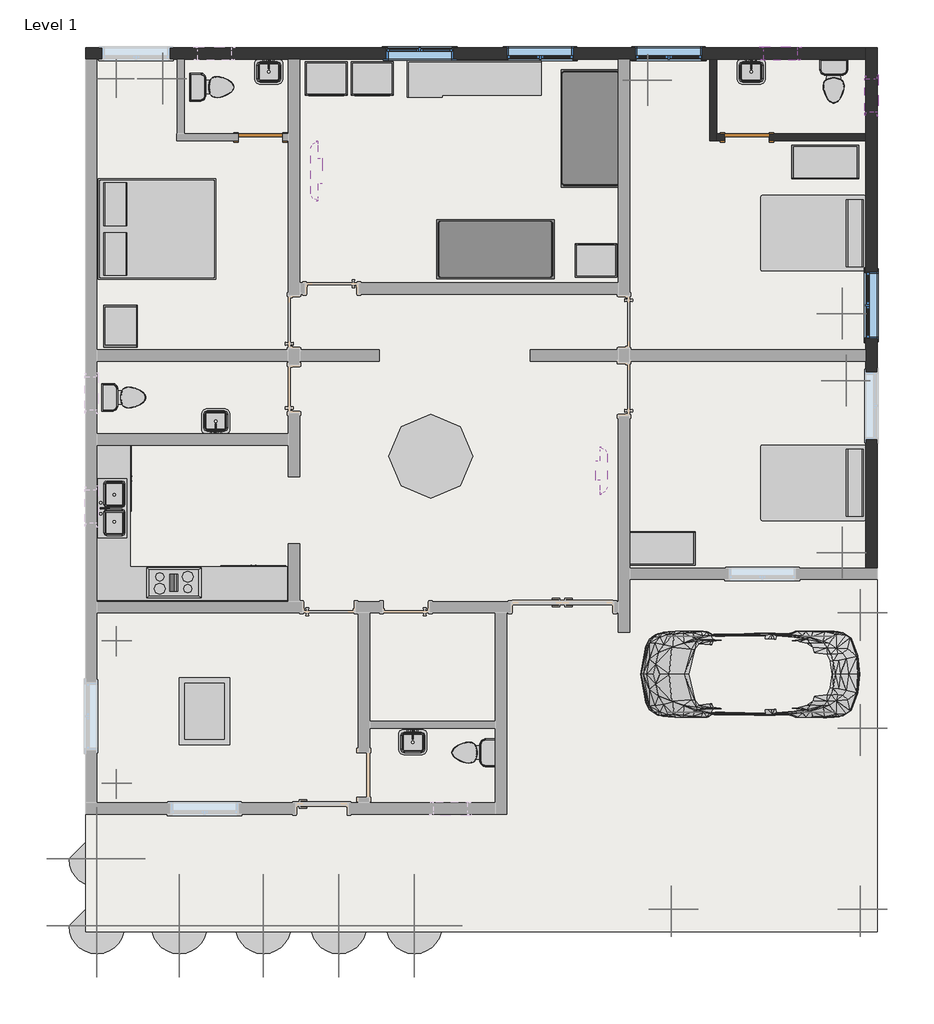
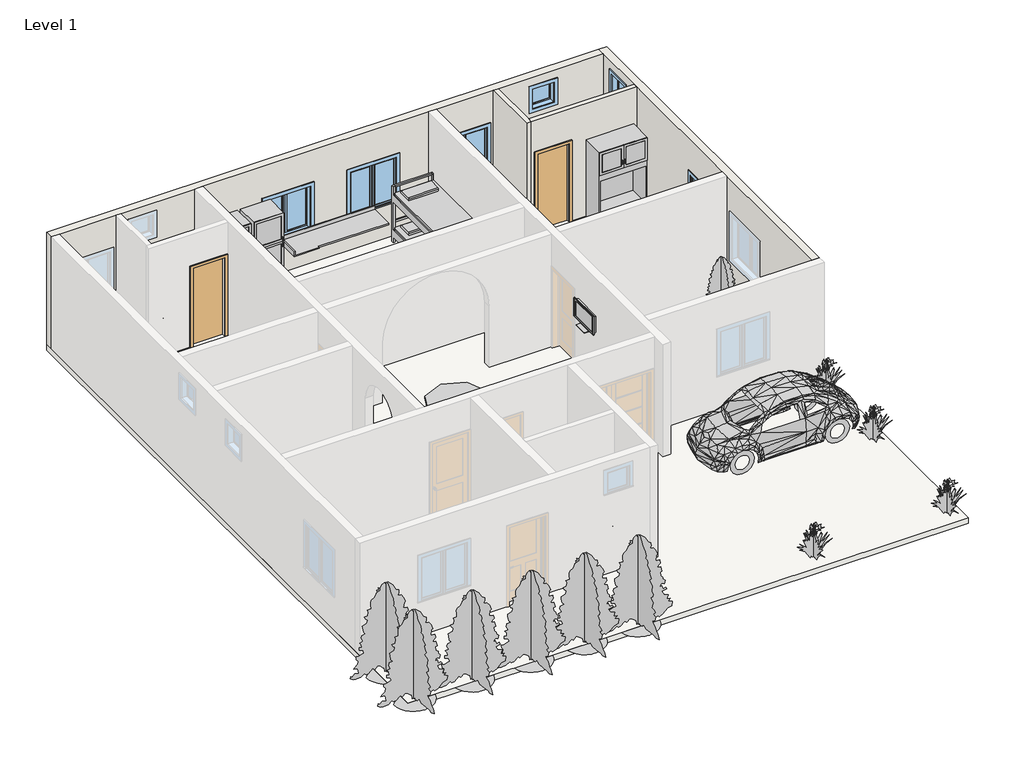
# One storey, part 2 of 2: 20 furniture elements, 18 geographic elements, 9 flow terminals, 6 windows, 4 walls, 2 doors, 2 proxies, 1 slab.
# Revit data of these elements (continued)
# Element 25 (IfcFurniture, "TV - Flat Screen : 42\"")
#   Stand = yes
#   Phase Created = New Construction
#   Materials on its faces: "TV - Black", "TV - Glass", "TV - Screen"
# Element 26 (IfcFurniture, "Table-Coffee : 24\" x 24\" x 24\"")
#   Phase Created = New Construction
#   Materials on its faces: "Glass - Clear, Grey"
# Element 27 (IfcFurniture, "Table-Dining Round w Chairs : 36\" Diameter")
#   Phase Created = New Construction
#   Materials on its faces: "Pine", "Laminate, Linen, Matte"
# Element 28 (IfcFurniture, "Tall Cabinet-2 Door-Built in : 3'")
#   Phase Created = New Construction
#   Materials on its faces: "Cabinets", "Cabinets - Handles", "Glass"
# Elements 29, 30 (IfcFurniture, "Tall Cabinet-2 Door-Built in : 30\"")
#   Phase Created = New Construction
#   Materials on its faces: "Cabinets", "Cabinets - Handles", "Glass"
# Elements 31, 32, 33 (IfcFurniture, "Tall Cabinet-Single Door(2) : 30\"")
#   Phase Created = New Construction
#   Materials on its faces: "Cabinets", "Cabinets - Handles"
# Elements 34, 35, 36, 37 (IfcGeographicElement, "RPC Plant - Tropical")
#   Phase Created = New Construction
# Elements 38, 39, 40, 41, 42, 43 (IfcGeographicElement, "RPC Tree - Conifer")
#   Phase Created = New Construction
# Element 44 (IfcGeographicElement, "RPC Tree - Conifer : 8'")
#   Phase Created = New Construction
# Elements 45, 46 (IfcGeographicElement, "RPC Tree - Conifer : Chinese Juniper - 7'")
#   Phase Created = New Construction
# Element 47 (IfcGeographicElement, "RPC Tree - Conifer : Eastern Hemlock - 25'")
#   Phase Created = New Construction
# Element 48 (IfcGeographicElement, "RPC Tree - Conifer : r")
#   Phase Created = New Construction
# Elements 49, 50 (IfcGeographicElement, "RPC Tree - Conifer : t")
#   Phase Created = New Construction
# Element 51 (IfcGeographicElement, "RPC Tree - Conifer : y")
#   Phase Created = New Construction
# Element 52 (IfcSlab, "Generic - 12\"")
#   Height Offset From Level = 0' - 0"
#   Phase Created = New Construction
#   Materials on its faces: "Oak Flooring"
# Elements 53, 54 (IfcWall, "Generic - 5\"")
#   Top Offset = 0' - 0"
#   Base Offset = 0' - 0"
#   Unconnected Height = 10' - 0"
#   wall height = 10' - 0"
#   Phase Created = New Construction
#   Base Constraint = Level 1
#   Materials on its faces: "Default Wall"
# Element 55 (IfcWall, "Generic - 8\"")
#   Top Offset = 0' - 0"
#   Base Offset = 0' - 0"
#   Unconnected Height = 10' - 0"
#   wall height = 10' - 0"
#   Phase Created = New Construction
#   Base Constraint = Level 1
#   Materials on its faces: "Paint - Sienna", "Default Wall"
# Element 56 (IfcWall, "Generic - 8\"")
#   Top Offset = 0' - 0"
#   Base Offset = 0' - 0"
#   Unconnected Height = 10' - 0"
#   wall height = 10' - 0"
#   Phase Created = New Construction
#   Base Constraint = Level 1
#   Materials on its faces: "Paint - Sienna"
# Element 57 (IfcWindow, "Casement Dbl with Trim : 48\" x 48\"")
#   Mark = "2"
#   Phase Created = New Construction
#   Materials on its faces: "Sash", "Trim", "Glass"
# Element 58 (IfcWindow, "Casement Dbl with Trim : 48\" x 48\"")
#   Mark = "3"
#   Phase Created = New Construction
#   Materials on its faces: "Sash", "Trim", "Glass"
# Element 59 (IfcWindow, "Casement Dbl with Trim : 48\" x 48\"")
#   Mark = "4"
#   Phase Created = New Construction
#   Materials on its faces: "Sash", "Trim", "Glass"
# Element 60 (IfcWindow, "Casement Dbl with Trim : 48\" x 48\"")
#   Mark = "5"
#   Phase Created = New Construction
#   Materials on its faces: "Sash", "Trim", "Glass"
# Element 61 (IfcWindow, "Transom with Trim : 24\" x 24\"")
#   Mark = "12"
#   Phase Created = New Construction
#   Materials on its faces: "Sash", "Trim", "Glass"
# Element 62 (IfcWindow, "Transom with Trim : 24\" x 24\"")
#   Mark = "13"
#   Phase Created = New Construction
#   Materials on its faces: "Sash", "Trim", "Glass"
# Materials
#   "Steel, Chrome Plated": class "Metal", colour RGB 17 17 17, transparency 0, Description = "Chromiuim plated steel", Cost = 0
#   "Steel, Polished": class "Metal", colour RGB 192 192 192, transparency 0, Description = "Polished steel", Cost = 0
#   "Wood - Birch - Solid Stained Light Low Gloss": class "Wood", colour RGB 210 159 95, transparency 0, Cost = 0
#   "Paint - Sienna": colour RGB 118 70 51, transparency 0, Cost = 0
#   "Porcelain, Linen": class "Ceramic", colour RGB 249 239 230, transparency 0, Description = "Porcelain, linen", Cost = 0
#   "Laminate, Linen, Matte": class "Plastic", colour RGB 249 239 230, transparency 0, Description = "Plastic Laminate - Linen, Matte", Cost = 0
#   "Cabinets - Handles": class "Metal", colour RGB 57 57 57, transparency 0
#   "Birch": class "Wood", colour RGB 224 178 126, transparency 0, Description = "Betula Alleghaniensis", Cost = 0
#   "Linen, White": class "Textile", colour RGB 247 247 239, transparency 0, Description = "Linen, white", Cost = 0
#   "Pine": class "Wood", colour RGB 223 192 134, transparency 0, Description = "Pinus Echinata", Cost = 0
#   "Glass": class "Glass", colour RGB 0 128 192, transparency 0.75, Description = "Soda Lime Glass", Cost = 0
#   "Oak Flooring": class "Wood", colour RGB 216 169 114, transparency 0, Description = "Quercus Rubra", Cost = 0
#   "Sash": class "Wood", colour RGB 224 178 126, transparency 0
#   "Trim": class "Wood", colour RGB 224 178 126, transparency 0
#   "Cabinets": colour RGB 249 249 249, transparency 0
#   "Counter Top": class "Wood", colour RGB 226 177 128, transparency 0
#   "TV - Black": colour RGB 49 49 49, transparency 0
#   "TV - Glass": colour RGB 157 157 157, transparency 0.9
#   "TV - Screen": colour RGB 0 0 0, transparency 0
#   "Glass - Clear, Grey": class "Glass", colour RGB 252 255 255, transparency 0.64
#   "Default Wall": colour RGB 128 128 128, transparency 0
